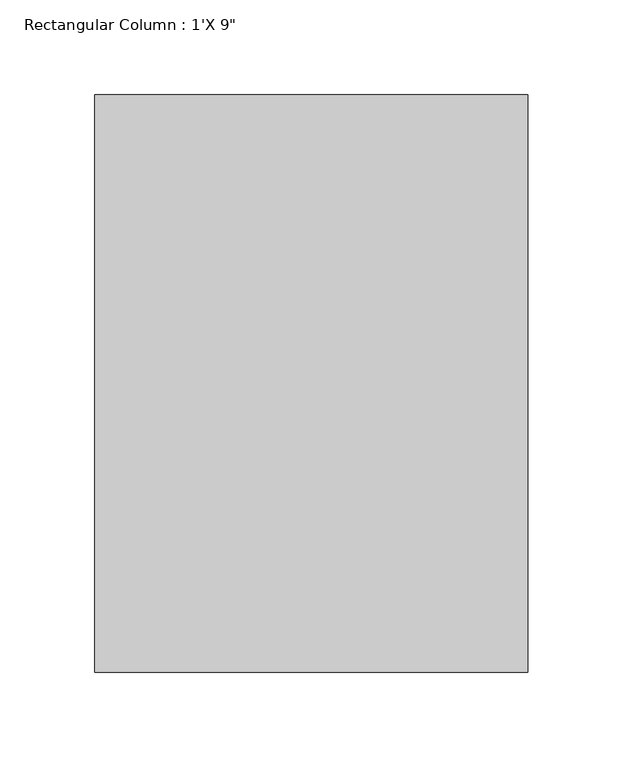
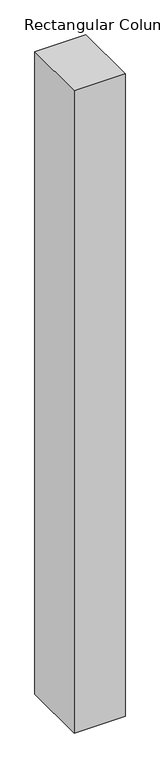
"""IFC4 building model written with IfcOpenShell, lengths in millimetres: column geometry."""

from ifc_helpers import new_model, si_unit, frame, origin, place, context, project, spatial, polyline, outline, extrude, source, transform, mapped, element, save


def column_f8de5b68(model_context):
    return source(origin(), model_context, "Body", "SweptSolid", [
        extrude(outline(polyline([(114.3, 152.4), (114.3, -152.4), (-114.3, -152.4), (-114.3, 152.4), (114.3, 152.4)])), frame((0.0, 0.0, 25603.2), z_axis=(0.0, 0.0, 1.0), x_axis=(1.0, 0.0, 0.0)), (0.0, 0.0, 1.0), 3048.0),
    ])


if __name__ == "__main__":
    model = new_model("IFC4")
    model_context = context("Model", 3, world=origin())
    ifc_project = project(units=[si_unit("LENGTHUNIT", "METRE", prefix="MILLI")], contexts=[model_context])
    site = spatial("IfcSite", under=ifc_project)
    building = spatial("IfcBuilding", under=site)
    placement = place(None, origin())
    column_shape = column_f8de5b68(model_context)
    element("IfcColumn", 1, ObjectType="Rectangular Column : 1'X 9\"", at=placement, inside=building, context=model_context, shape_type="MappedRepresentation", body=[
        mapped(column_shape, transform((0.0, 0.0, 0.0), x_axis=(1.0, 0.0, 0.0), y_axis=(0.0, 1.0, 0.0), z_axis=(0.0, 0.0, 1.0))),
    ])
    save(model, "model.ifc")

# Revit data of these elements
# Type "Rectangular Column : 1'X 9\""
#   Assembly Code = "B1010200"
#   Depth = 1' - 0"
#   Offset Base = 0' - 0"
#   Offset Top = 0' - 0"
#   Width = 0' - 9"
#   Material = none
